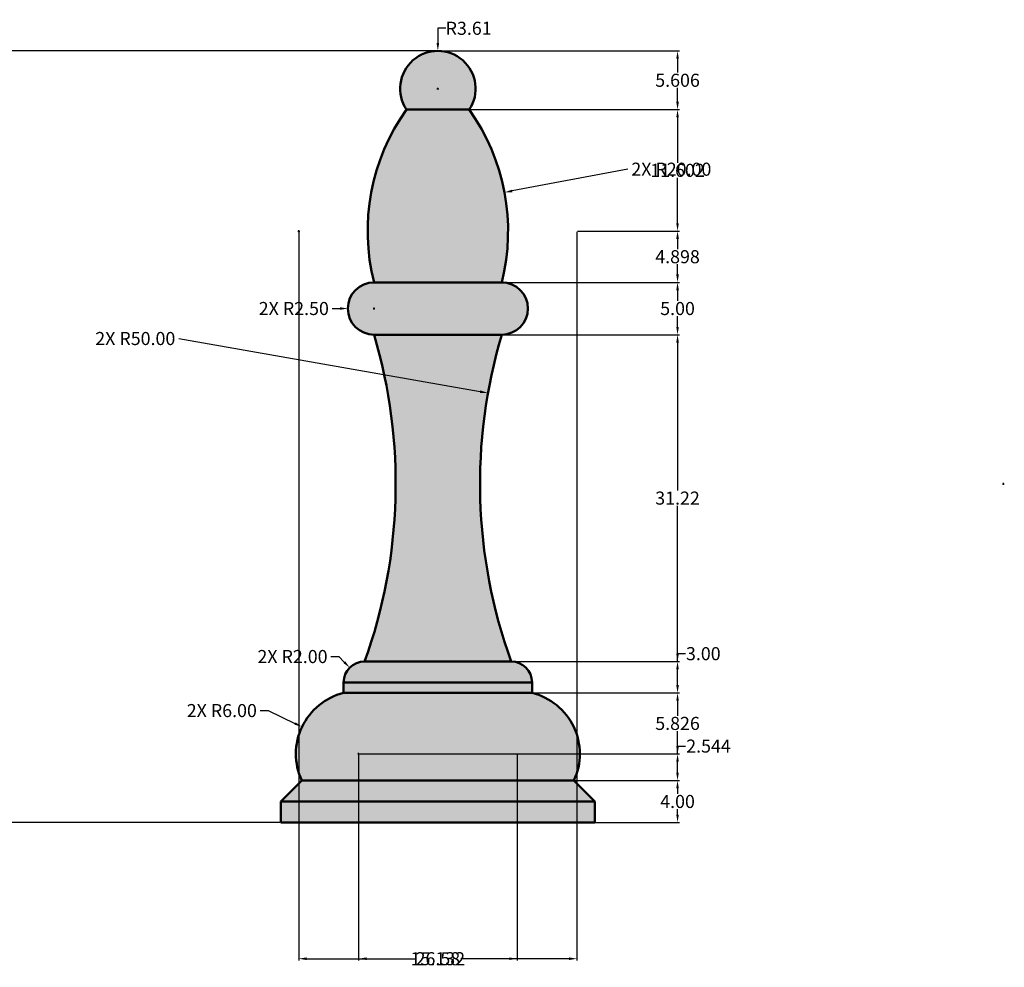
# Model space of a CAD drawing. Units: millimetres. Extents: x 184 to 390, y 95 to 263.
# Tile 2 of 2: x 296 to 390, y 95 to 186. Entities that reach past the tile are written whole.
import ezdxf

# ---------------------------------------------------------------- set-up
doc = ezdxf.new("R2010")
doc.units = ezdxf.units.MM
doc.header["$MEASUREMENT"] = 0
for name, color, linetype, lineweight in [('M-DIMS', 2, 'Continuous', 25), ('M-HATC', 8, 'Continuous', 18), ('M-OUTL', 7, 'Continuous', 50)]:
    doc.layers.add(name, color=color, linetype=linetype, lineweight=lineweight)
doc.styles.get("Standard").update_dxf_attribs({"font": 'arial.ttf'})
doc.dimstyles.get("Standard").update_dxf_attribs({"dimtxt": 1.25, "dimasz": 0.75, "dimexe": 0.18, "dimexo": 0.0625, "dimgap": 0.09, "dimtad": 0, "dimtih": 1, "dimtoh": 1, "dimdec": 0, "dimzin": 0, "dimdsep": 46, "dimtxsty": 'Standard', "dimcen": 0.09, "dimadec": 0, "dimazin": 0, "dimtfac": 1, "dimtdec": 0, "dimtofl": 0, "dimtmove": 0, "dimatfit": 3, "dimfxl": 1, "dimtolj": 1, "dimtzin": 0, "dimarcsym": 0})

# ---------------------------------------------------------------- blocks, each defined once
blk = doc.blocks.new('*D42')
at = {"layer": 'Defpoints', "color": 0, "transparency": 16777216}
for p in [(328.535, 115.528), (343.667, 115.528), (343.667, 95.964)]:
    blk.add_point(p, dxfattribs=at)
at = {"layer": 'M-DIMS', "color": 0, "lineweight": -2, "transparency": 16777216}
for p, q in [((328.535, 115.465), (328.535, 95.784)), ((343.667, 115.465), (343.667, 95.784)), ((329.285, 95.964), (333.482, 95.964)), ((342.917, 95.964), (338.72, 95.964))]:
    blk.add_line(p, q, dxfattribs=at)
at = {"layer": 'M-DIMS', "color": 0, "transparency": 16777216}
for points in [[(329.285, 96.089), (329.285, 95.839), (328.535, 95.964)], [(342.917, 96.089), (342.917, 95.839), (343.667, 95.964)]]:
    blk.add_solid(points, dxfattribs=at)
at = {"layer": 'M-DIMS', "color": 0, "transparency": 16777216, "insert": (336.101, 95.964), "char_height": 1.25, "attachment_point": 5}
blk.add_mtext('\\A1;15.132', dxfattribs=at)
blk = doc.blocks.new('*D43')
at = {"layer": 'Defpoints', "color": 0, "transparency": 16777216}
for p in [(322.81, 165.472), (349.392, 165.472), (349.392, 95.964)]:
    blk.add_point(p, dxfattribs=at)
at = {"layer": 'M-DIMS', "color": 0, "lineweight": -2, "transparency": 16777216}
for p, q in [((322.81, 165.41), (322.81, 95.784)), ((349.392, 165.41), (349.392, 95.784)), ((323.56, 95.964), (333.89, 95.964)), ((348.642, 95.964), (338.312, 95.964))]:
    blk.add_line(p, q, dxfattribs=at)
at = {"layer": 'M-DIMS', "color": 0, "transparency": 16777216}
for points in [[(323.56, 96.089), (323.56, 95.839), (322.81, 95.964)], [(348.642, 96.089), (348.642, 95.839), (349.392, 95.964)]]:
    blk.add_solid(points, dxfattribs=at)
at = {"layer": 'M-DIMS', "color": 0, "transparency": 16777216, "insert": (336.101, 95.964), "char_height": 1.25, "attachment_point": 5}
blk.add_mtext('\\A1;26.58', dxfattribs=at)
blk = doc.blocks.new('*D44')
at = {"layer": 'Defpoints', "color": 0, "transparency": 16777216}
for p in [(336.101, 112.984), (359.001, 112.984), (336.101, 108.984)]:
    blk.add_point(p, dxfattribs=at)
at = {"layer": 'M-DIMS', "color": 0, "lineweight": -2, "transparency": 16777216}
for p, q in [((336.163, 112.984), (359.181, 112.984)), ((359.001, 112.234), (359.001, 111.712)), ((359.001, 109.734), (359.001, 110.256)), ((336.163, 108.984), (359.181, 108.984))]:
    blk.add_line(p, q, dxfattribs=at)
at = {"layer": 'M-DIMS', "color": 0, "transparency": 16777216}
for points in [[(358.876, 112.234), (359.126, 112.234), (359.001, 112.984)], [(358.876, 109.734), (359.126, 109.734), (359.001, 108.984)]]:
    blk.add_solid(points, dxfattribs=at)
at = {"layer": 'M-DIMS', "color": 0, "transparency": 16777216, "insert": (359.001, 110.984), "char_height": 1.25, "attachment_point": 5}
blk.add_mtext('\\A1;4.00', dxfattribs=at)
blk = doc.blocks.new('*D45')
at = {"layer": 'Defpoints', "color": 0, "transparency": 16777216}
for p in [(328.535, 115.528), (359.001, 115.528), (336.101, 112.984)]:
    blk.add_point(p, dxfattribs=at)
at = {"layer": 'M-DIMS', "color": 0, "lineweight": -2, "transparency": 16777216}
for p, q in [((359.001, 115.528), (359.001, 116.278)), ((359.001, 116.278), (359.751, 116.278)), ((328.598, 115.528), (359.181, 115.528)), ((359.001, 113.734), (359.001, 114.778)), ((336.163, 112.984), (359.181, 112.984))]:
    blk.add_line(p, q, dxfattribs=at)
at = {"layer": 'M-DIMS', "color": 0, "transparency": 16777216}
for points in [[(358.876, 114.778), (359.126, 114.778), (359.001, 115.528)], [(358.876, 113.734), (359.126, 113.734), (359.001, 112.984)]]:
    blk.add_solid(points, dxfattribs=at)
at = {"layer": 'M-DIMS', "color": 0, "transparency": 16777216, "insert": (361.958, 116.278), "char_height": 1.25, "attachment_point": 5}
blk.add_mtext('\\A1;2.544', dxfattribs=at)
blk = doc.blocks.new('*D46')
at = {"layer": 'Defpoints', "color": 0, "transparency": 16777216}
for p in [(345.101, 121.354), (359.001, 121.354), (328.535, 115.528)]:
    blk.add_point(p, dxfattribs=at)
at = {"layer": 'M-DIMS', "color": 0, "lineweight": -2, "transparency": 16777216}
for p, q in [((345.163, 121.354), (359.181, 121.354)), ((359.001, 120.604), (359.001, 119.169)), ((359.001, 116.278), (359.001, 117.713)), ((328.598, 115.528), (359.181, 115.528))]:
    blk.add_line(p, q, dxfattribs=at)
at = {"layer": 'M-DIMS', "color": 0, "transparency": 16777216}
for points in [[(358.876, 120.604), (359.126, 120.604), (359.001, 121.354)], [(358.876, 116.278), (359.126, 116.278), (359.001, 115.528)]]:
    blk.add_solid(points, dxfattribs=at)
at = {"layer": 'M-DIMS', "color": 0, "transparency": 16777216, "insert": (359.001, 118.441), "char_height": 1.25, "attachment_point": 5}
blk.add_mtext('\\A1;5.826', dxfattribs=at)
blk = doc.blocks.new('*D47')
at = {"layer": 'Defpoints', "color": 0, "transparency": 16777216}
for p in [(343.101, 124.354), (359.001, 124.354), (345.101, 121.354)]:
    blk.add_point(p, dxfattribs=at)
at = {"layer": 'M-DIMS', "color": 0, "lineweight": -2, "transparency": 16777216}
for p, q in [((343.163, 124.354), (359.181, 124.354)), ((359.001, 124.354), (359.001, 125.104)), ((359.001, 125.104), (359.751, 125.104)), ((359.001, 122.104), (359.001, 123.604)), ((345.163, 121.354), (359.181, 121.354))]:
    blk.add_line(p, q, dxfattribs=at)
at = {"layer": 'M-DIMS', "color": 0, "transparency": 16777216}
for points in [[(358.876, 123.604), (359.126, 123.604), (359.001, 124.354)], [(358.876, 122.104), (359.126, 122.104), (359.001, 121.354)]]:
    blk.add_solid(points, dxfattribs=at)
at = {"layer": 'M-DIMS', "color": 0, "transparency": 16777216, "insert": (361.462, 125.104), "char_height": 1.25, "attachment_point": 5}
blk.add_mtext('\\A1;3.00', dxfattribs=at)
blk = doc.blocks.new('*D48')
at = {"layer": 'Defpoints', "color": 0, "transparency": 16777216}
for p in [(342.201, 155.574), (359.001, 155.574), (343.101, 124.354)]:
    blk.add_point(p, dxfattribs=at)
at = {"layer": 'M-DIMS', "color": 0, "lineweight": -2, "transparency": 16777216}
for p, q in [((342.263, 155.574), (359.181, 155.574)), ((359.001, 154.824), (359.001, 140.693)), ((359.001, 125.104), (359.001, 139.235)), ((343.163, 124.354), (359.181, 124.354))]:
    blk.add_line(p, q, dxfattribs=at)
at = {"layer": 'M-DIMS', "color": 0, "transparency": 16777216}
for points in [[(358.876, 154.824), (359.126, 154.824), (359.001, 155.574)], [(358.876, 125.104), (359.126, 125.104), (359.001, 124.354)]]:
    blk.add_solid(points, dxfattribs=at)
at = {"layer": 'M-DIMS', "color": 0, "transparency": 16777216, "insert": (359.001, 139.964), "char_height": 1.25, "attachment_point": 5}
blk.add_mtext('\\A1;31.22', dxfattribs=at)
blk = doc.blocks.new('*D49')
at = {"layer": 'Defpoints', "color": 0, "transparency": 16777216}
for p in [(342.201, 160.574), (359.001, 160.574), (342.201, 155.574)]:
    blk.add_point(p, dxfattribs=at)
at = {"layer": 'M-DIMS', "color": 0, "lineweight": -2, "transparency": 16777216}
for p, q in [((342.263, 160.574), (359.181, 160.574)), ((359.001, 159.824), (359.001, 158.802)), ((359.001, 156.324), (359.001, 157.346)), ((342.263, 155.574), (359.181, 155.574))]:
    blk.add_line(p, q, dxfattribs=at)
at = {"layer": 'M-DIMS', "color": 0, "transparency": 16777216}
for points in [[(358.876, 159.824), (359.126, 159.824), (359.001, 160.574)], [(358.876, 156.324), (359.126, 156.324), (359.001, 155.574)]]:
    blk.add_solid(points, dxfattribs=at)
at = {"layer": 'M-DIMS', "color": 0, "transparency": 16777216, "insert": (359.001, 158.074), "char_height": 1.25, "attachment_point": 5}
blk.add_mtext('\\A1;5.00', dxfattribs=at)
blk = doc.blocks.new('*D50')
at = {"layer": 'Defpoints', "color": 0, "transparency": 16777216}
for p in [(349.392, 165.472), (359.001, 165.472), (342.201, 160.574)]:
    blk.add_point(p, dxfattribs=at)
at = {"layer": 'M-DIMS', "color": 0, "lineweight": -2, "transparency": 16777216}
for p, q in [((349.454, 165.472), (359.181, 165.472)), ((359.001, 164.722), (359.001, 163.751)), ((359.001, 161.324), (359.001, 162.295)), ((342.263, 160.574), (359.181, 160.574))]:
    blk.add_line(p, q, dxfattribs=at)
at = {"layer": 'M-DIMS', "color": 0, "transparency": 16777216}
for points in [[(358.876, 164.722), (359.126, 164.722), (359.001, 165.472)], [(358.876, 161.324), (359.126, 161.324), (359.001, 160.574)]]:
    blk.add_solid(points, dxfattribs=at)
at = {"layer": 'M-DIMS', "color": 0, "transparency": 16777216, "insert": (359.001, 163.023), "char_height": 1.25, "attachment_point": 5}
blk.add_mtext('\\A1;4.898', dxfattribs=at)
blk = doc.blocks.new('*D51')
at = {"layer": 'Defpoints', "color": 0, "transparency": 16777216}
for p in [(339.101, 177.074), (359.001, 177.074), (349.392, 165.472)]:
    blk.add_point(p, dxfattribs=at)
at = {"layer": 'M-DIMS', "color": 0, "lineweight": -2, "transparency": 16777216}
for p, q in [((339.163, 177.074), (359.181, 177.074)), ((359.001, 176.324), (359.001, 172.001)), ((359.001, 166.222), (359.001, 170.545)), ((349.454, 165.472), (359.181, 165.472))]:
    blk.add_line(p, q, dxfattribs=at)
at = {"layer": 'M-DIMS', "color": 0, "transparency": 16777216}
for points in [[(358.876, 176.324), (359.126, 176.324), (359.001, 177.074)], [(358.876, 166.222), (359.126, 166.222), (359.001, 165.472)]]:
    blk.add_solid(points, dxfattribs=at)
at = {"layer": 'M-DIMS', "color": 0, "transparency": 16777216, "insert": (359.001, 171.273), "char_height": 1.25, "attachment_point": 5}
blk.add_mtext('\\A1;11.602', dxfattribs=at)
blk = doc.blocks.new('*D52')
at = {"layer": 'Defpoints', "color": 0, "transparency": 16777216}
for p in [(336.101, 182.68), (359.001, 182.68), (339.101, 177.074)]:
    blk.add_point(p, dxfattribs=at)
at = {"layer": 'M-DIMS', "color": 0, "lineweight": -2, "transparency": 16777216}
for p, q in [((336.163, 182.68), (359.181, 182.68)), ((359.001, 181.93), (359.001, 180.605)), ((359.001, 177.824), (359.001, 179.149)), ((339.163, 177.074), (359.181, 177.074))]:
    blk.add_line(p, q, dxfattribs=at)
at = {"layer": 'M-DIMS', "color": 0, "transparency": 16777216}
for points in [[(358.876, 181.93), (359.126, 181.93), (359.001, 182.68)], [(358.876, 177.824), (359.126, 177.824), (359.001, 177.074)]]:
    blk.add_solid(points, dxfattribs=at)
at = {"layer": 'M-DIMS', "color": 0, "transparency": 16777216, "insert": (359.001, 179.877), "char_height": 1.25, "attachment_point": 5}
blk.add_mtext('\\A1;5.606', dxfattribs=at)
blk = doc.blocks.new('*D53')
at = {"layer": 'Defpoints', "color": 0, "transparency": 16777216}
for p in [(210.188, 182.68), (336.101, 182.68), (321.101, 108.984)]:
    blk.add_point(p, dxfattribs=at)
at = {"layer": 'M-DIMS', "color": 0, "lineweight": -2, "transparency": 16777216}
for p, q in [((336.038, 182.68), (210.008, 182.68)), ((210.188, 181.93), (210.188, 146.561)), ((210.188, 109.734), (210.188, 145.103)), ((321.038, 108.984), (210.008, 108.984))]:
    blk.add_line(p, q, dxfattribs=at)
at = {"layer": 'M-DIMS', "color": 0, "transparency": 16777216}
for points in [[(210.063, 181.93), (210.313, 181.93), (210.188, 182.68)], [(210.063, 109.734), (210.313, 109.734), (210.188, 108.984)]]:
    blk.add_solid(points, dxfattribs=at)
at = {"layer": 'M-DIMS', "color": 0, "transparency": 16777216, "insert": (210.188, 145.832), "char_height": 1.25, "attachment_point": 5}
blk.add_mtext('\\A1;73.70', dxfattribs=at)
blk = doc.blocks.new('*D54')
at = {"layer": 'Defpoints', "color": 0, "transparency": 16777216}
for p in [(342.466, 169.165), (322.81, 165.472)]:
    blk.add_point(p, dxfattribs=at)
at = {"layer": 'M-DIMS', "color": 0, "lineweight": -2, "transparency": 16777216}
for p, q in [((354.26, 171.381), (343.203, 169.304)), ((322.72, 165.472), (322.9, 165.472)), ((322.81, 165.382), (322.81, 165.562))]:
    blk.add_line(p, q, dxfattribs=at)
at = {"layer": 'M-DIMS', "color": 0, "transparency": 16777216}
blk.add_solid([(343.18, 169.426), (343.226, 169.181), (342.466, 169.165)], dxfattribs=at)
at = {"layer": 'M-DIMS', "color": 0, "transparency": 16777216, "insert": (358.408, 171.381), "char_height": 1.25, "attachment_point": 5}
blk.add_mtext('\\A1;2X R20.00', dxfattribs=at)
blk = doc.blocks.new('*D55')
at = {"layer": 'Defpoints', "color": 0, "transparency": 16777216}
for p in [(323.121, 118.115), (328.535, 115.528)]:
    blk.add_point(p, dxfattribs=at)
at = {"layer": 'M-DIMS', "color": 0, "lineweight": -2, "transparency": 16777216}
for p, q in [((319.123, 119.667), (319.873, 119.667)), ((319.873, 119.667), (322.445, 118.438)), ((328.445, 115.528), (328.625, 115.528)), ((328.535, 115.438), (328.535, 115.618))]:
    blk.add_line(p, q, dxfattribs=at)
at = {"layer": 'M-DIMS', "color": 0, "transparency": 16777216}
blk.add_solid([(322.499, 118.551), (322.391, 118.325), (323.121, 118.115)], dxfattribs=at)
at = {"layer": 'M-DIMS', "color": 0, "transparency": 16777216, "insert": (315.46, 119.667), "char_height": 1.25, "attachment_point": 5}
blk.add_mtext('\\A1;2X R6.00', dxfattribs=at)
blk = doc.blocks.new('*D56')
at = {"layer": 'Defpoints', "color": 0, "transparency": 16777216}
for p in [(340.888, 150.004), (390.13, 141.333)]:
    blk.add_point(p, dxfattribs=at)
at = {"layer": 'M-DIMS', "color": 0, "lineweight": -2, "transparency": 16777216}
for p, q in [((311.342, 155.207), (340.149, 150.134)), ((390.04, 141.333), (390.22, 141.333)), ((390.13, 141.243), (390.13, 141.423))]:
    blk.add_line(p, q, dxfattribs=at)
at = {"layer": 'M-DIMS', "color": 0, "transparency": 16777216}
blk.add_solid([(340.171, 150.257), (340.127, 150.011), (340.888, 150.004)], dxfattribs=at)
at = {"layer": 'M-DIMS', "color": 0, "transparency": 16777216, "insert": (307.194, 155.207), "char_height": 1.25, "attachment_point": 5}
blk.add_mtext('\\A1;2X R50.00', dxfattribs=at)
blk = doc.blocks.new('*D57')
at = {"layer": 'Defpoints', "color": 0, "transparency": 16777216}
for p in [(336.101, 182.68), (336.101, 179.074)]:
    blk.add_point(p, dxfattribs=at)
at = {"layer": 'M-DIMS', "color": 0, "lineweight": -2, "transparency": 16777216}
for p, q in [((336.851, 184.843), (336.101, 184.843)), ((336.101, 184.843), (336.101, 183.43)), ((336.011, 179.074), (336.191, 179.074)), ((336.101, 178.984), (336.101, 179.164))]:
    blk.add_line(p, q, dxfattribs=at)
at = {"layer": 'M-DIMS', "color": 0, "transparency": 16777216}
blk.add_solid([(335.976, 183.43), (336.226, 183.43), (336.101, 182.68)], dxfattribs=at)
at = {"layer": 'M-DIMS', "color": 0, "transparency": 16777216, "insert": (339.042, 184.843), "char_height": 1.25, "attachment_point": 5}
blk.add_mtext('\\A1;R3.61', dxfattribs=at)
blk = doc.blocks.new('*D58')
at = {"layer": 'Defpoints', "color": 0, "transparency": 16777216}
for p in [(327.501, 158.074), (330.001, 158.074)]:
    blk.add_point(p, dxfattribs=at)
at = {"layer": 'M-DIMS', "color": 0, "lineweight": -2, "transparency": 16777216}
for p, q in [((326.001, 158.074), (326.751, 158.074)), ((329.911, 158.074), (330.091, 158.074)), ((330.001, 157.984), (330.001, 158.164))]:
    blk.add_line(p, q, dxfattribs=at)
at = {"layer": 'M-DIMS', "color": 0, "transparency": 16777216}
blk.add_solid([(326.751, 158.199), (326.751, 157.949), (327.501, 158.074)], dxfattribs=at)
at = {"layer": 'M-DIMS', "color": 0, "transparency": 16777216, "insert": (322.338, 158.074), "char_height": 1.25, "attachment_point": 5}
blk.add_mtext('\\A1;2X R2.50', dxfattribs=at)
blk = doc.blocks.new('*D59')
at = {"layer": 'Defpoints', "color": 0, "transparency": 16777216}
for p in [(327.687, 123.768), (329.101, 122.354)]:
    blk.add_point(p, dxfattribs=at)
at = {"layer": 'M-DIMS', "color": 0, "lineweight": -2, "transparency": 16777216}
for p, q in [((325.876, 124.829), (326.626, 124.829)), ((326.626, 124.829), (327.156, 124.299)), ((329.011, 122.354), (329.191, 122.354)), ((329.101, 122.264), (329.101, 122.444))]:
    blk.add_line(p, q, dxfattribs=at)
at = {"layer": 'M-DIMS', "color": 0, "transparency": 16777216}
blk.add_solid([(327.245, 124.387), (327.068, 124.21), (327.687, 123.768)], dxfattribs=at)
at = {"layer": 'M-DIMS', "color": 0, "transparency": 16777216, "insert": (322.213, 124.829), "char_height": 1.25, "attachment_point": 5}
blk.add_mtext('\\A1;2X R2.00', dxfattribs=at)

msp = doc.modelspace()

# ---------------------------------------------------------------- hatches: boundary and pattern name
at = {"layer": 'M-HATC'}
h = msp.add_hatch(color=256, dxfattribs=at)
h.dxf.hatch_style = 1
h.paths.add_polyline_path([(339.101, 177.0741), (336.101, 177.0741), (333.101, 177.0741, 0.2200173), (330.001, 160.5741), (336.101, 160.5741), (342.201, 160.5741, 0.2200173)])
h.paths.add_polyline_path([(342.201, 160.5741), (336.101, 160.5741), (330.001, 160.5741, 1), (330.001, 155.5741), (336.101, 155.5741), (342.201, 155.5741, 1)])
h.paths.add_polyline_path([(342.201, 155.5741), (336.101, 155.5741), (330.001, 155.5741, -0.1601712), (329.101, 124.3541), (343.101, 124.3541, -0.1601712)])
h.paths.add_polyline_path([(345.101, 121.3541), (336.101, 121.3541), (327.101, 121.3541, 0.4730098), (323.101, 112.9841), (336.101, 112.9841), (349.101, 112.9841, 0.4730098)])
h.paths.add_polyline_path([(345.101, 122.3541), (327.101, 122.3541), (327.101, 121.3541), (336.101, 121.3541), (345.101, 121.3541)])
h.paths.add_polyline_path([(343.101, 124.3541), (329.101, 124.3541, 0.4142136), (327.101, 122.3541), (345.101, 122.3541, 0.4142136)])
h.paths.add_polyline_path([(349.101, 112.9841), (336.101, 112.9841), (323.101, 112.9841), (321.101, 110.9841), (351.101, 110.9841)])
h.paths.add_polyline_path([(351.101, 110.9841), (321.101, 110.9841), (321.101, 108.9841), (336.101, 108.9841), (351.101, 108.9841)])
h.paths.add_polyline_path([(333.101, 177.0741), (336.101, 177.0741), (339.101, 177.0741, 1.8685171)])

# ---------------------------------------------------------------- linework, layer by layer
at = {"layer": 'M-OUTL'}
for p, q in [((336.101, 177.0741), (333.101, 177.0741)), ((336.101, 177.0741), (334.9671, 177.0741)), ((336.101, 177.0741), (337.2349, 177.0741)), ((336.101, 177.0741), (339.101, 177.0741)), ((330.001, 160.5741), (336.101, 160.5741)), ((342.201, 160.5741), (336.101, 160.5741)), ((336.101, 155.5741), (330.001, 155.5741)), ((336.101, 155.5741), (330.001, 155.5741)), ((336.101, 155.5741), (342.201, 155.5741)), ((329.101, 124.3541), (343.101, 124.3541)), ((327.101, 121.3541), (327.101, 122.3541)), ((327.101, 122.3541), (345.101, 122.3541)), ((345.101, 122.3541), (345.101, 121.3541)), ((336.101, 121.3541), (327.101, 121.3541)), ((336.101, 121.3541), (345.101, 121.3541)), ((323.101, 112.9841), (321.101, 110.9841)), ((323.101, 112.9841), (336.101, 112.9841)), ((349.101, 112.9841), (336.101, 112.9841)), ((349.101, 112.9841), (351.101, 110.9841)), ((351.101, 110.9841), (321.101, 110.9841)), ((321.101, 110.9841), (321.101, 108.9841)), ((351.101, 108.9841), (351.101, 110.9841)), ((321.101, 108.9841), (336.101, 108.9841)), ((336.101, 108.9841), (351.101, 108.9841))]:
    msp.add_line(p, q, dxfattribs=at)
for centre, radius, start, end in [((336.101, 179.0741), 3.6056, 326.309932, 213.690068), ((349.3919, 165.4722), 20, 144.542648, 194.176113), ((322.81, 165.4722), 20, 345.823887, 35.457352), ((330.001, 158.0741), 2.5, 90, 270), ((342.201, 158.0741), 2.5, 270, 90), ((282.072, 141.3328), 50, 340.149068, 16.548438), ((390.13, 141.3328), 50, 163.451562, 199.850932), ((329.101, 122.3541), 2, 90, 180), ((343.101, 122.3541), 2, 0, 90), ((328.535, 115.528), 6, 103.827775, 205.086211), ((343.667, 115.528), 6, 334.913789, 76.172225)]:
    msp.add_arc(centre, radius, start, end, dxfattribs=at)

# ---------------------------------------------------------------- dimensions: what is measured, and where the dimension line sits
at = {"layer": 'M-DIMS'}
dim = msp.add_radius_dim(center=(336.101, 179.0741), mpoint=(336.101, 182.6796), dimstyle='Standard', override={"dimdec": 2, "dimlfac": 1, "dimrnd": 0, "dimzin": 0, "dimdsep": 46, "dimlunit": 2}, dxfattribs=at)
dim.commit()
dim.dimension.update_dxf_attribs({"geometry": '*D57', "text_midpoint": (339.042, 184.843), "dimtype": 164})
for base, p1, p2, override, picture, middle in [((210.1879, 182.6796), (321.101, 108.9841), (336.101, 182.6796), {"dimdec": 2, "dimlfac": 1, "dimrnd": 0, "dimzin": 0, "dimdsep": 46, "dimlunit": 2}, '*D53', (210.1879, 145.8319)), ((359.001, 182.67964), (339.101, 177.07409), (336.101, 182.67964), {"dimdec": 3, "dimlfac": 1, "dimrnd": 0, "dimzin": 0, "dimdsep": 46, "dimlunit": 2}, '*D52', (359.001, 179.87687)), ((359.001, 177.0741), (349.3919, 165.4722), (339.101, 177.0741), {"dimdec": 3, "dimlfac": 1, "dimrnd": 0, "dimzin": 0, "dimdsep": 46, "dimlunit": 2}, '*D51', (359.001, 171.2731)), ((359.001, 165.4722), (342.201, 160.5741), (349.3919, 165.4722), {"dimdec": 3, "dimlfac": 1, "dimrnd": 0, "dimzin": 0, "dimdsep": 46, "dimlunit": 2}, '*D50', (359.001, 163.0231)), ((359.001, 160.5741), (342.201, 155.5741), (342.201, 160.5741), {"dimdec": 2, "dimlfac": 1, "dimrnd": 0, "dimzin": 0, "dimdsep": 46, "dimlunit": 2}, '*D49', (359.001, 158.0741)), ((359.001, 155.5741), (343.101, 124.3541), (342.201, 155.5741), {"dimdec": 2, "dimlfac": 1, "dimrnd": 0, "dimzin": 0, "dimdsep": 46, "dimlunit": 2}, '*D48', (359.001, 139.9641)), ((359.001, 124.3541), (345.101, 121.3541), (343.101, 124.3541), {"dimdec": 2, "dimlfac": 1, "dimrnd": 0, "dimzin": 0, "dimdsep": 46, "dimlunit": 2}, '*D47', (361.4619, 125.1041)), ((359.001, 121.3541), (328.535, 115.528), (345.101, 121.3541), {"dimdec": 3, "dimlfac": 1, "dimrnd": 0, "dimzin": 0, "dimdsep": 46, "dimlunit": 2}, '*D46', (359.001, 118.441)), ((359.001, 115.528), (336.101, 112.9841), (328.535, 115.528), {"dimdec": 3, "dimlfac": 1, "dimrnd": 0, "dimzin": 0, "dimdsep": 46, "dimlunit": 2}, '*D45', (361.9582, 116.278)), ((359.001, 112.9841), (336.101, 108.9841), (336.101, 112.9841), {"dimdec": 2, "dimlfac": 1, "dimrnd": 0, "dimzin": 0, "dimdsep": 46, "dimlunit": 2}, '*D44', (359.001, 110.9841))]:
    dim = msp.add_linear_dim(base=base, p1=p1, p2=p2, angle=90, dimstyle='Standard', override=override, dxfattribs=at)
    dim.commit()
    dim.dimension.update_dxf_attribs({"geometry": picture, "text_midpoint": middle})
for center, mpoint, picture, middle in [((322.81, 165.4722), (342.4662, 169.165), '*D54', (354.2598, 171.3808)), ((390.13, 141.3328), (340.8876, 150.0039), '*D56', (311.3422, 155.2066)), ((328.535, 115.528), (323.1213, 118.1148), '*D55', (315.46, 119.667))]:
    dim = msp.add_radius_dim(center=center, mpoint=mpoint, text='2X <>', dimstyle='Standard', override={"dimdec": 2, "dimlfac": 1, "dimrnd": 0, "dimzin": 0, "dimdsep": 46, "dimlunit": 2}, dxfattribs=at)
    dim.commit()
    dim.dimension.update_dxf_attribs({"geometry": picture, "text_midpoint": middle, "dimtype": 164})
for base, p1, p2, override, picture in [((349.3919, 95.9641), (322.81, 165.4722), (349.3919, 165.4722), {"dimdec": 2, "dimlfac": 1, "dimrnd": 0, "dimzin": 0, "dimdsep": 46, "dimlunit": 2}, '*D43'), ((343.667, 95.9641), (328.535, 115.528), (343.667, 115.528), {"dimdec": 3, "dimlfac": 1, "dimrnd": 0, "dimzin": 0, "dimdsep": 46, "dimlunit": 2}, '*D42')]:
    dim = msp.add_linear_dim(base=base, p1=p1, p2=p2, dimstyle='Standard', override=override, dxfattribs=at)
    dim.commit()
    dim.dimension.update_dxf_attribs({"geometry": picture, "text_midpoint": (336.101, 95.9641)})
for center, mpoint, picture, middle in [((330.001, 158.0741), (327.501, 158.074), '*D58', (326.001, 158.0739)), ((329.101, 122.3541), (327.6867, 123.7683), '*D59', (322.213, 124.8289))]:
    dim = msp.add_radius_dim(center=center, mpoint=mpoint, text='2X <>', dimstyle='Standard', override={"dimdec": 2, "dimlfac": 1, "dimrnd": 0, "dimzin": 0, "dimdsep": 46, "dimlunit": 2}, dxfattribs=at)
    dim.commit()
    dim.dimension.update_dxf_attribs({"geometry": picture, "text_midpoint": middle})

doc.saveas('drawing.dxf')
